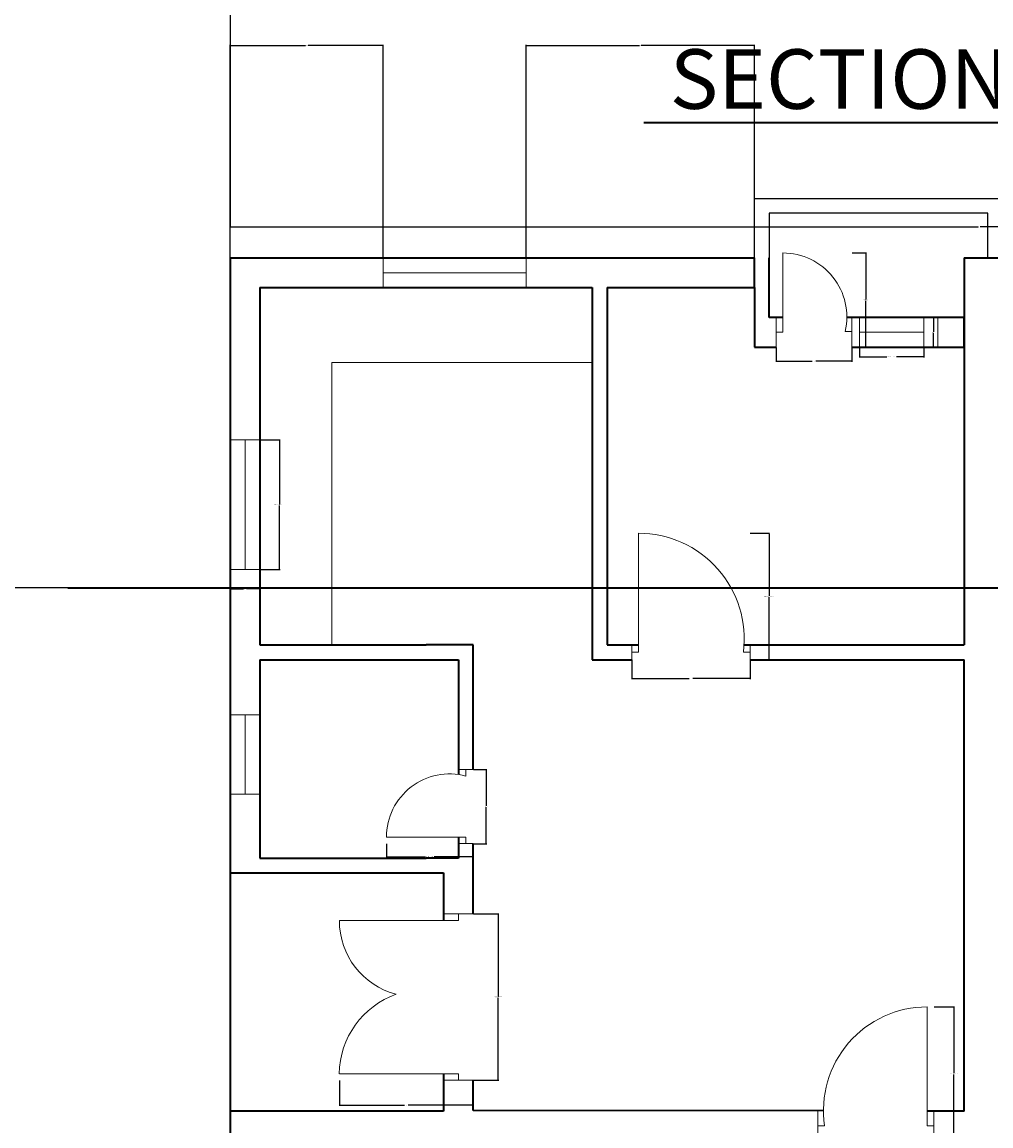
# Model space of a CAD drawing. Units: inches. Extents: x 2250 to 3629, y 982 to 2740.
# Tile 8 of 12: x 2918 to 3211, y 1785 to 2119. Entities that reach past the tile are written whole.
import ezdxf

# ---------------------------------------------------------------- set-up
doc = ezdxf.new("R2010")
doc.units = ezdxf.units.IN
for name, color, linetype, lineweight in [('A-ANNO-DIMS', 2, 'Continuous', 18), ('A-ANNO-SYMB', 7, 'Continuous', 35), ('A-ANNO-TITL', 7, 'Continuous', 35), ('A-DOOR', 3, 'Continuous', 18), ('A-FLOR-DECK', 7, 'Continuous', 25), ('A-FLOR-FIXT', 9, 'Continuous', 18), ('A-GLAZ', 4, 'Continuous', 18), ('A-WALL', 7, 'Continuous', 35)]:
    doc.layers.add(name, color=color, linetype=linetype, lineweight=lineweight)
doc.styles.get("Standard").update_dxf_attribs({"font": 'arial.ttf'})
doc.dimstyles.get("Standard").update_dxf_attribs({"dimtxt": 0.18, "dimasz": 0.18, "dimexe": 0.18, "dimexo": 0.0625, "dimgap": 0.09, "dimtad": 0, "dimtih": 1, "dimtoh": 1, "dimdec": 4, "dimzin": 0, "dimdsep": 46, "dimtxsty": 'Standard', "dimcen": 0.09, "dimadec": 0, "dimazin": 0, "dimtfac": 1, "dimtdec": 4, "dimtofl": 0, "dimtmove": 0, "dimatfit": 3, "dimfxl": 1, "dimtolj": 1, "dimtzin": 0, "dimarcsym": 0})

# ---------------------------------------------------------------- blocks, each defined once
blk = doc.blocks.new('DR-36-BED-NW')
for p, q in [((2, 2.25), (2, 38.25)), ((0, 4.5), (0, 0)), ((35.76, 4.5), (35.76, 0)), ((0, 0), (0, 2.25)), ((0, 2.25), (2, 2.25)), ((35.76, 2.25), (33.76, 2.25)), ((35.76, 0), (35.76, 2.25))]:
    blk.add_line(p, q)
blk.add_arc((2, 6.24), 32.01, 352.8376, 90)
blk = doc.blocks.new('DR-24-DECK-NW')
for p, q in [((2, 4.5), (2, 28.5)), ((0, 9), (0, 0)), ((22.88, 0), (22.88, 9)), ((22.88, 9), (22.88, 4.79)), ((0, 0), (0, 4.5)), ((0, 4.5), (2, 4.5)), ((22.88, 4.79), (20.88, 4.79))]:
    blk.add_line(p, q)
blk.add_arc((2, 9.13), 19.37, 347.0543, 90)
blk = doc.blocks.new('DR-72-DECK-WEST-N')
for p, q in [((31.5, 50.33), (40.5, 50.33)), ((40.5, 50.33), (36, 50.33)), ((36, 50.33), (36, 48.33)), ((36, 48.33), (0, 48.33)), ((36, 2), (0, 2)), ((36, 0), (36, 2)), ((31.5, 0), (40.5, 0)), ((40.5, 0), (36, 0))]:
    blk.add_line(p, q)
for centre, radius, start, end in [((23.09, 48.33), 23.09, 180, 255.1842), ((25.75, 1.72), 25.76, 109.4277, 179.3734)]:
    blk.add_arc(centre, radius, start, end)
blk = doc.blocks.new('DR-24-BATH-NW')
for p, q in [((21.75, 22.45), (26.25, 22.45)), ((26.25, 22.45), (24, 22.45)), ((24, 22.45), (24, 20.45)), ((24, 2), (0, 2)), ((24, 0), (24, 2)), ((21.75, 0), (26.25, 0)), ((26.25, 0), (24, 0))]:
    blk.add_line(p, q)
blk.add_arc((19.09, 2), 19.09, 75.0892, 180)
blk = doc.blocks.new('DR-36-ENTRY-NW')
for p, q in [((33.05, 4.5), (33.05, 40.5)), ((0, 9.04), (0, 0)), ((35.05, 9.01), (35.05, 0)), ((0, 0), (0, 4.52)), ((0, 4.52), (2, 4.52)), ((35.05, 4.5), (33.05, 4.5)), ((35.05, 0), (35.05, 4.5))]:
    blk.add_line(p, q)
blk.add_arc((33.05, 9.12), 31.39, 90, 188.415)
blk = doc.blocks.new('WIN-DECK-NW')
for p, q in [((0.07, 4.5), (0.07, 9)), ((0.07, 9), (0.07, 1.12)), ((19.52, 9), (19.52, 0)), ((19.52, 4.5), (0.07, 4.5)), ((19.52, 0), (19.52, 4.5)), ((0.07, 1.12), (0, 0))]:
    blk.add_line(p, q)
blk = doc.blocks.new('WIN-KITCHEN-NW-A')
for p, q in [((0, 9), (0, 0)), ((43.24, 4.5), (43.24, 9)), ((43.24, 9), (43.24, 0)), ((0, 4.5), (43.24, 4.5))]:
    blk.add_line(p, q)
blk = doc.blocks.new('WIN-KITCHEN-NW-B')
for p, q in [((0, 39.2), (9, 39.2)), ((4.5, 0), (4.5, 39.2)), ((9, 0), (0, 0)), ((0, 0), (4.5, 0))]:
    blk.add_line(p, q)
blk = doc.blocks.new('WIN-24-BATH-NW')
for p, q in [((9, 24), (0, 24)), ((0, 24), (4.5, 24)), ((4.5, 24), (4.5, 0)), ((9, 0), (0, 0)), ((4.5, 0), (9, 0))]:
    blk.add_line(p, q)
blk = doc.blocks.new('*D85')
at = {"layer": 'A-ANNO-DIMS', "color": 0, "lineweight": -2, "transparency": 16777216}
for p, q in [((3171.49, 2020.67), (3171.49, 2017.63)), ((3191.01, 2020.67), (3191.01, 2017.63)), ((3171.67, 2017.81), (3179.76, 2017.81)), ((3190.83, 2017.81), (3182.75, 2017.81))]:
    blk.add_line(p, q, dxfattribs=at)
at = {"layer": 'A-ANNO-DIMS', "color": 0, "transparency": 16777216}
for points in [[(3171.67, 2017.84), (3171.67, 2017.78), (3171.49, 2017.81)], [(3190.83, 2017.84), (3190.83, 2017.78), (3191.01, 2017.81)]]:
    blk.add_solid(points, dxfattribs=at)
at = {"layer": 'Defpoints', "color": 0, "transparency": 16777216}
for p in [(3171.49, 2020.74), (3191.01, 2020.74), (3191.01, 2017.81)]:
    blk.add_point(p, dxfattribs=at)
at = {"layer": 'A-ANNO-DIMS', "color": 0, "transparency": 16777216, "insert": (3181.25, 2017.81), "char_height": 0.18, "attachment_point": 5}
blk.add_mtext('\\A1;DECK WINDOW 20 TYP.', dxfattribs=at)
blk = doc.blocks.new('*D86')
at = {"layer": 'A-ANNO-DIMS', "color": 0, "lineweight": -2, "transparency": 16777216}
for p, q in [((3191.07, 2029.74), (3194.12, 2029.74)), ((3193.94, 2029.56), (3193.94, 2025.42)), ((3193.94, 2020.92), (3193.94, 2025.05)), ((3191.07, 2020.74), (3194.12, 2020.74))]:
    blk.add_line(p, q, dxfattribs=at)
at = {"layer": 'A-ANNO-DIMS', "color": 0, "transparency": 16777216}
for points in [[(3193.91, 2029.56), (3193.97, 2029.56), (3193.94, 2029.74)], [(3193.91, 2020.92), (3193.97, 2020.92), (3193.94, 2020.74)]]:
    blk.add_solid(points, dxfattribs=at)
at = {"layer": 'Defpoints', "color": 0, "transparency": 16777216}
for p in [(3191.01, 2029.74), (3193.94, 2029.74), (3191.01, 2020.74)]:
    blk.add_point(p, dxfattribs=at)
at = {"layer": 'A-ANNO-DIMS', "color": 0, "transparency": 16777216, "insert": (3193.94, 2025.24), "char_height": 0.18, "attachment_point": 5}
blk.add_mtext('\\A1;9 TYP.', dxfattribs=at)
blk = doc.blocks.new('*D89')
at = {"layer": 'A-ANNO-DIMS', "color": 0, "lineweight": -2, "transparency": 16777216}
for p, q in [((2990.29, 1992.69), (2996.29, 1992.69)), ((2996.11, 1992.51), (2996.11, 1973.27)), ((2996.11, 1953.67), (2996.11, 1972.9)), ((2990.29, 1953.49), (2996.29, 1953.49))]:
    blk.add_line(p, q, dxfattribs=at)
at = {"layer": 'A-ANNO-DIMS', "color": 0, "transparency": 16777216}
for points in [[(2996.08, 1992.51), (2996.14, 1992.51), (2996.11, 1992.69)], [(2996.08, 1953.67), (2996.14, 1953.67), (2996.11, 1953.49)]]:
    blk.add_solid(points, dxfattribs=at)
at = {"layer": 'Defpoints', "color": 0, "transparency": 16777216}
for p in [(2990.23, 1992.69), (2996.11, 1992.69), (2990.23, 1953.49)]:
    blk.add_point(p, dxfattribs=at)
at = {"layer": 'A-ANNO-DIMS', "color": 0, "transparency": 16777216, "insert": (2996.11, 1973.09), "char_height": 0.18, "attachment_point": 5}
blk.add_mtext('\\A1;KITCHEN WINDOW 39 TYP.', dxfattribs=at)
blk = doc.blocks.new('*D90')
at = {"layer": 'A-ANNO-DIMS', "color": 0, "lineweight": -2, "transparency": 16777216}
for p, q in [((2981.23, 1953.42), (2981.23, 1947.43)), ((2990.23, 1953.42), (2990.23, 1947.43)), ((2981.41, 1947.61), (2985.27, 1947.61)), ((2990.05, 1947.61), (2986.18, 1947.61))]:
    blk.add_line(p, q, dxfattribs=at)
at = {"layer": 'A-ANNO-DIMS', "color": 0, "transparency": 16777216}
for points in [[(2981.41, 1947.64), (2981.41, 1947.58), (2981.23, 1947.61)], [(2990.05, 1947.64), (2990.05, 1947.58), (2990.23, 1947.61)]]:
    blk.add_solid(points, dxfattribs=at)
at = {"layer": 'Defpoints', "color": 0, "transparency": 16777216}
for p in [(2981.23, 1953.49), (2990.23, 1953.49), (2990.23, 1947.61)]:
    blk.add_point(p, dxfattribs=at)
at = {"layer": 'A-ANNO-DIMS', "color": 0, "transparency": 16777216, "insert": (2985.73, 1947.61), "char_height": 0.18, "attachment_point": 5}
blk.add_mtext('\\A1;9 TYP.', dxfattribs=at)
blk = doc.blocks.new('*D103')
at = {"layer": 'A-ANNO-DIMS', "color": 0, "lineweight": -2, "transparency": 16777216}
for p, q in [((3138.49, 1964.49), (3144.35, 1964.49)), ((3144.17, 1964.31), (3144.17, 1945.54)), ((3144.17, 1926.42), (3144.17, 1945.18)), ((3138.49, 1926.24), (3144.35, 1926.24))]:
    blk.add_line(p, q, dxfattribs=at)
at = {"layer": 'A-ANNO-DIMS', "color": 0, "transparency": 16777216}
for points in [[(3144.14, 1964.31), (3144.2, 1964.31), (3144.17, 1964.49)], [(3144.14, 1926.42), (3144.2, 1926.42), (3144.17, 1926.24)]]:
    blk.add_solid(points, dxfattribs=at)
at = {"layer": 'Defpoints', "color": 0, "transparency": 16777216}
for p in [(3138.43, 1964.49), (3144.17, 1964.49), (3138.43, 1926.24)]:
    blk.add_point(p, dxfattribs=at)
at = {"layer": 'A-ANNO-DIMS', "color": 0, "transparency": 16777216, "insert": (3144.17, 1945.36), "char_height": 0.18, "attachment_point": 5}
blk.add_mtext('\\A1;BEDROOM DOOR 38 TYP.', dxfattribs=at)
blk = doc.blocks.new('*D104')
at = {"layer": 'A-ANNO-DIMS', "color": 0, "lineweight": -2, "transparency": 16777216}
for p, q in [((3102.67, 1926.17), (3102.67, 1920.32)), ((3138.43, 1926.17), (3138.43, 1920.32)), ((3102.85, 1920.5), (3120.02, 1920.5)), ((3138.25, 1920.5), (3121.08, 1920.5))]:
    blk.add_line(p, q, dxfattribs=at)
at = {"layer": 'A-ANNO-DIMS', "color": 0, "transparency": 16777216}
for points in [[(3102.85, 1920.53), (3102.85, 1920.47), (3102.67, 1920.5)], [(3138.25, 1920.53), (3138.25, 1920.47), (3138.43, 1920.5)]]:
    blk.add_solid(points, dxfattribs=at)
at = {"layer": 'Defpoints', "color": 0, "transparency": 16777216}
for p in [(3102.67, 1926.24), (3138.43, 1926.24), (3138.43, 1920.5)]:
    blk.add_point(p, dxfattribs=at)
at = {"layer": 'A-ANNO-DIMS', "color": 0, "transparency": 16777216, "insert": (3120.55, 1920.5), "char_height": 0.18, "attachment_point": 5}
blk.add_mtext('\\A1;36 TYP.', dxfattribs=at)
blk = doc.blocks.new('*D105')
at = {"layer": 'A-ANNO-DIMS', "color": 0, "lineweight": -2, "transparency": 16777216}
for p, q in [((3169.27, 2049.24), (3173.67, 2049.24)), ((3173.49, 2049.06), (3173.49, 2035.17)), ((3173.49, 2020.92), (3173.49, 2034.8)), ((3169.27, 2020.74), (3173.67, 2020.74))]:
    blk.add_line(p, q, dxfattribs=at)
at = {"layer": 'A-ANNO-DIMS', "color": 0, "transparency": 16777216}
for points in [[(3173.46, 2049.06), (3173.52, 2049.06), (3173.49, 2049.24)], [(3173.46, 2020.92), (3173.52, 2020.92), (3173.49, 2020.74)]]:
    blk.add_solid(points, dxfattribs=at)
at = {"layer": 'Defpoints', "color": 0, "transparency": 16777216}
for p in [(3169.21, 2049.24), (3173.49, 2049.24), (3169.21, 2020.74)]:
    blk.add_point(p, dxfattribs=at)
at = {"layer": 'A-ANNO-DIMS', "color": 0, "transparency": 16777216, "insert": (3173.49, 2034.99), "char_height": 0.18, "attachment_point": 5}
blk.add_mtext('\\A1;DECK DOOR 29 TYP.', dxfattribs=at)
blk = doc.blocks.new('*D106')
at = {"layer": 'A-ANNO-DIMS', "color": 0, "lineweight": -2, "transparency": 16777216}
for p, q in [((3146.34, 2020.67), (3146.34, 2016.28)), ((3169.21, 2020.67), (3169.21, 2016.28)), ((3146.52, 2016.46), (3157.24, 2016.46)), ((3169.03, 2016.46), (3158.3, 2016.46))]:
    blk.add_line(p, q, dxfattribs=at)
at = {"layer": 'A-ANNO-DIMS', "color": 0, "transparency": 16777216}
for points in [[(3146.52, 2016.49), (3146.52, 2016.43), (3146.34, 2016.46)], [(3169.03, 2016.49), (3169.03, 2016.43), (3169.21, 2016.46)]]:
    blk.add_solid(points, dxfattribs=at)
at = {"layer": 'Defpoints', "color": 0, "transparency": 16777216}
for p in [(3146.34, 2020.74), (3169.21, 2020.74), (3169.21, 2016.46)]:
    blk.add_point(p, dxfattribs=at)
at = {"layer": 'A-ANNO-DIMS', "color": 0, "transparency": 16777216, "insert": (3157.77, 2016.46), "char_height": 0.18, "attachment_point": 5}
blk.add_mtext('\\A1;23 TYP.', dxfattribs=at)
blk = doc.blocks.new('*D107')
at = {"layer": 'A-ANNO-DIMS', "color": 0, "lineweight": -2, "transparency": 16777216}
for p, q in [((3054.79, 1849.36), (3062.46, 1849.36)), ((3062.28, 1849.18), (3062.28, 1824.38)), ((3062.28, 1799.21), (3062.28, 1824.01)), ((3054.79, 1799.03), (3062.46, 1799.03))]:
    blk.add_line(p, q, dxfattribs=at)
at = {"layer": 'A-ANNO-DIMS', "color": 0, "transparency": 16777216}
for points in [[(3062.25, 1849.18), (3062.31, 1849.18), (3062.28, 1849.36)], [(3062.25, 1799.21), (3062.31, 1799.21), (3062.28, 1799.03)]]:
    blk.add_solid(points, dxfattribs=at)
at = {"layer": 'Defpoints', "color": 0, "transparency": 16777216}
for p in [(3054.73, 1849.36), (3062.28, 1849.36), (3054.73, 1799.03)]:
    blk.add_point(p, dxfattribs=at)
at = {"layer": 'A-ANNO-DIMS', "color": 0, "transparency": 16777216, "insert": (3062.28, 1824.2), "char_height": 0.18, "attachment_point": 5}
blk.add_mtext('\\A1;DECK DOOR 50 TYP.', dxfattribs=at)
blk = doc.blocks.new('*D108')
at = {"layer": 'A-ANNO-DIMS', "color": 0, "lineweight": -2, "transparency": 16777216}
for p, q in [((3014.23, 1798.97), (3014.23, 1791.3)), ((3054.73, 1798.97), (3054.73, 1791.3)), ((3014.41, 1791.48), (3033.95, 1791.48)), ((3054.55, 1791.48), (3035.01, 1791.48))]:
    blk.add_line(p, q, dxfattribs=at)
at = {"layer": 'A-ANNO-DIMS', "color": 0, "transparency": 16777216}
for points in [[(3014.41, 1791.51), (3014.41, 1791.45), (3014.23, 1791.48)], [(3054.55, 1791.51), (3054.55, 1791.45), (3054.73, 1791.48)]]:
    blk.add_solid(points, dxfattribs=at)
at = {"layer": 'Defpoints', "color": 0, "transparency": 16777216}
for p in [(3014.23, 1799.03), (3054.73, 1799.03), (3054.73, 1791.48)]:
    blk.add_point(p, dxfattribs=at)
at = {"layer": 'A-ANNO-DIMS', "color": 0, "transparency": 16777216, "insert": (3034.48, 1791.48), "char_height": 0.18, "attachment_point": 5}
blk.add_mtext('\\A1;41 TYP.', dxfattribs=at)
blk = doc.blocks.new('*D109')
at = {"layer": 'A-ANNO-DIMS', "color": 0, "lineweight": -2, "transparency": 16777216}
for p, q in [((3028.48, 1870.53), (3028.48, 1866.48)), ((3054.73, 1870.53), (3054.73, 1866.48)), ((3028.66, 1866.66), (3040.3, 1866.66)), ((3054.55, 1866.66), (3042.91, 1866.66))]:
    blk.add_line(p, q, dxfattribs=at)
at = {"layer": 'A-ANNO-DIMS', "color": 0, "transparency": 16777216}
for points in [[(3028.66, 1866.69), (3028.66, 1866.63), (3028.48, 1866.66)], [(3054.55, 1866.69), (3054.55, 1866.63), (3054.73, 1866.66)]]:
    blk.add_solid(points, dxfattribs=at)
at = {"layer": 'Defpoints', "color": 0, "transparency": 16777216}
for p in [(3028.48, 1870.59), (3054.73, 1870.59), (3054.73, 1866.66)]:
    blk.add_point(p, dxfattribs=at)
at = {"layer": 'A-ANNO-DIMS', "color": 0, "transparency": 16777216, "insert": (3041.6, 1866.66), "char_height": 0.18, "attachment_point": 5}
blk.add_mtext('\\A1;BATH DOOR 26 TYP.', dxfattribs=at)
blk = doc.blocks.new('*D110')
at = {"layer": 'A-ANNO-DIMS', "color": 0, "lineweight": -2, "transparency": 16777216}
for p, q in [((3054.79, 1893.04), (3058.84, 1893.04)), ((3058.66, 1892.86), (3058.66, 1882)), ((3058.66, 1870.77), (3058.66, 1881.64)), ((3054.79, 1870.59), (3058.84, 1870.59))]:
    blk.add_line(p, q, dxfattribs=at)
at = {"layer": 'A-ANNO-DIMS', "color": 0, "transparency": 16777216}
for points in [[(3058.63, 1892.86), (3058.69, 1892.86), (3058.66, 1893.04)], [(3058.63, 1870.77), (3058.69, 1870.77), (3058.66, 1870.59)]]:
    blk.add_solid(points, dxfattribs=at)
at = {"layer": 'Defpoints', "color": 0, "transparency": 16777216}
for p in [(3054.73, 1893.04), (3058.66, 1893.04), (3054.73, 1870.59)]:
    blk.add_point(p, dxfattribs=at)
at = {"layer": 'A-ANNO-DIMS', "color": 0, "transparency": 16777216, "insert": (3058.66, 1881.82), "char_height": 0.18, "attachment_point": 5}
blk.add_mtext('\\A1;22 TYP.', dxfattribs=at)
blk = doc.blocks.new('*D137')
at = {"layer": 'A-ANNO-DIMS', "color": 0, "lineweight": -2, "transparency": 16777216}
for p, q in [((3194.07, 1821.24), (3200.27, 1821.24)), ((3200.09, 1821.06), (3200.09, 1801.17)), ((3200.09, 1780.92), (3200.09, 1800.8)), ((3194.07, 1780.74), (3200.27, 1780.74))]:
    blk.add_line(p, q, dxfattribs=at)
at = {"layer": 'A-ANNO-DIMS', "color": 0, "transparency": 16777216}
for points in [[(3200.06, 1821.06), (3200.12, 1821.06), (3200.09, 1821.24)], [(3200.06, 1780.92), (3200.12, 1780.92), (3200.09, 1780.74)]]:
    blk.add_solid(points, dxfattribs=at)
at = {"layer": 'Defpoints', "color": 0, "transparency": 16777216}
for p in [(3194.01, 1821.24), (3200.09, 1821.24), (3194.01, 1780.74)]:
    blk.add_point(p, dxfattribs=at)
at = {"layer": 'A-ANNO-DIMS', "color": 0, "transparency": 16777216, "insert": (3200.09, 1800.99), "char_height": 0.18, "attachment_point": 5}
blk.add_mtext('\\A1;ENTRY DOOR 41 TYP.', dxfattribs=at)
blk = doc.blocks.new('*D172')
at = {"layer": 'A-ANNO-DIMS', "color": 0, "lineweight": -2, "transparency": 16777216}
for p, q in [((3433.02, 2070.24), (3541.21, 2070.24)), ((3541.03, 2070.06), (3541.03, 1664.67)), ((3541.03, 1258.92), (3541.03, 1664.3)), ((3059.29, 1258.74), (3541.21, 1258.74))]:
    blk.add_line(p, q, dxfattribs=at)
at = {"layer": 'A-ANNO-DIMS', "color": 0, "transparency": 16777216}
for points in [[(3541, 2070.06), (3541.06, 2070.06), (3541.03, 2070.24)], [(3541, 1258.92), (3541.06, 1258.92), (3541.03, 1258.74)]]:
    blk.add_solid(points, dxfattribs=at)
at = {"layer": 'Defpoints', "color": 0, "transparency": 16777216}
for p in [(3432.96, 2070.24), (3541.03, 2070.24), (3059.23, 1258.74)]:
    blk.add_point(p, dxfattribs=at)
at = {"layer": 'A-ANNO-DIMS', "color": 0, "transparency": 16777216, "insert": (3541.03, 1664.49), "char_height": 0.18, "attachment_point": 5}
blk.add_mtext('\\A1;811.5', dxfattribs=at)
blk = doc.blocks.new('*D173')
at = {"layer": 'A-ANNO-DIMS', "color": 0, "lineweight": -2, "transparency": 16777216}
for p, q in [((2932.01, 1947.92), (2890.14, 1947.92)), ((2890.32, 1947.74), (2890.32, 1603.51)), ((2890.32, 1258.92), (2890.32, 1603.15)), ((2981.16, 1258.74), (2890.14, 1258.74))]:
    blk.add_line(p, q, dxfattribs=at)
at = {"layer": 'A-ANNO-DIMS', "color": 0, "transparency": 16777216}
for points in [[(2890.29, 1947.74), (2890.35, 1947.74), (2890.32, 1947.92)], [(2890.29, 1258.92), (2890.35, 1258.92), (2890.32, 1258.74)]]:
    blk.add_solid(points, dxfattribs=at)
at = {"layer": 'Defpoints', "color": 0, "transparency": 16777216}
for p in [(2932.07, 1947.92), (2890.32, 1258.74), (2981.23, 1258.74)]:
    blk.add_point(p, dxfattribs=at)
at = {"layer": 'A-ANNO-DIMS', "color": 0, "transparency": 16777216, "insert": (2890.32, 1603.33), "char_height": 0.18, "attachment_point": 5}
blk.add_mtext('\\A1;689.2', dxfattribs=at)
blk = doc.blocks.new('*D174')
at = {"layer": 'A-ANNO-DIMS', "color": 0, "lineweight": -2, "transparency": 16777216}
for p, q in [((2981.23, 2047.8), (2981.23, 2112.17)), ((2981.41, 2111.99), (3003.97, 2111.99)), ((3027.33, 2111.99), (3004.77, 2111.99)), ((3027.51, 2047.8), (3027.51, 2112.17))]:
    blk.add_line(p, q, dxfattribs=at)
at = {"layer": 'A-ANNO-DIMS', "color": 0, "transparency": 16777216}
for points in [[(2981.41, 2112.02), (2981.41, 2111.96), (2981.23, 2111.99)], [(3027.33, 2112.02), (3027.33, 2111.96), (3027.51, 2111.99)]]:
    blk.add_solid(points, dxfattribs=at)
at = {"layer": 'Defpoints', "color": 0, "transparency": 16777216}
for p in [(3027.51, 2111.99), (2981.23, 2047.74), (3027.51, 2047.74)]:
    blk.add_point(p, dxfattribs=at)
at = {"layer": 'A-ANNO-DIMS', "color": 0, "transparency": 16777216, "insert": (3004.37, 2111.99), "char_height": 0.18, "attachment_point": 5}
blk.add_mtext('\\A1;46.29', dxfattribs=at)
blk = doc.blocks.new('*D175')
at = {"layer": 'A-ANNO-DIMS', "color": 0, "lineweight": -2, "transparency": 16777216}
for p, q in [((3070.76, 2047.8), (3070.76, 2112.17)), ((3070.94, 2111.99), (3105.04, 2111.99)), ((3139.57, 2111.99), (3105.47, 2111.99)), ((3139.75, 2047.8), (3139.75, 2112.17))]:
    blk.add_line(p, q, dxfattribs=at)
at = {"layer": 'A-ANNO-DIMS', "color": 0, "transparency": 16777216}
for points in [[(3070.94, 2112.02), (3070.94, 2111.96), (3070.76, 2111.99)], [(3139.57, 2112.02), (3139.57, 2111.96), (3139.75, 2111.99)]]:
    blk.add_solid(points, dxfattribs=at)
at = {"layer": 'Defpoints', "color": 0, "transparency": 16777216}
for p in [(3139.75, 2111.99), (3070.76, 2047.74), (3139.75, 2047.74)]:
    blk.add_point(p, dxfattribs=at)
at = {"layer": 'A-ANNO-DIMS', "color": 0, "transparency": 16777216, "insert": (3105.25, 2111.99), "char_height": 0.18, "attachment_point": 5}
blk.add_mtext('\\A1;69', dxfattribs=at)
blk = doc.blocks.new('*D188')
at = {"layer": 'A-ANNO-DIMS', "color": 0, "lineweight": -2, "transparency": 16777216}
for p, q in [((2981.23, 2131.64), (2981.23, 2056.9)), ((3434.23, 2131.64), (3434.23, 2056.9)), ((2981.41, 2057.08), (3207.43, 2057.08)), ((3434.05, 2057.08), (3208.02, 2057.08))]:
    blk.add_line(p, q, dxfattribs=at)
at = {"layer": 'A-ANNO-DIMS', "color": 0, "transparency": 16777216}
for points in [[(2981.41, 2057.11), (2981.41, 2057.05), (2981.23, 2057.08)], [(3434.05, 2057.11), (3434.05, 2057.05), (3434.23, 2057.08)]]:
    blk.add_solid(points, dxfattribs=at)
at = {"layer": 'Defpoints', "color": 0, "transparency": 16777216}
for p in [(2981.23, 2131.7), (3434.23, 2131.7), (3434.23, 2057.08)]:
    blk.add_point(p, dxfattribs=at)
at = {"layer": 'A-ANNO-DIMS', "color": 0, "transparency": 16777216, "insert": (3207.73, 2057.08), "char_height": 0.18, "attachment_point": 5}
blk.add_mtext('\\A1;453', dxfattribs=at)

msp = doc.modelspace()

# ---------------------------------------------------------------- linework, layer by layer
at = {"layer": 'A-ANNO-SYMB'}
msp.add_line((2932.0741, 1947.9231), (3499.2778, 1947.9231), dxfattribs=at)
at = {"layer": 'A-ANNO-TITL'}
msp.add_line((3253.0344, 2088.5817), (3106.2899, 2088.5817), dxfattribs=at)
at = {"layer": 'A-FLOR-DECK'}
for p, q in [((3139.754, 2047.7354), (3139.754, 2065.7354)), ((3139.754, 2065.7354), (3214.8276, 2065.7354)), ((3210.3276, 2061.2354), (3144.254, 2061.2354)), ((3144.254, 2061.2354), (3144.254, 2046.3774)), ((3210.3276, 2047.7354), (3210.3276, 2061.2354)), ((3214.8276, 2047.7354), (3210.3276, 2047.7354))]:
    msp.add_line(p, q, dxfattribs=at)
at = {"layer": 'A-FLOR-FIXT'}
for p, q in [((3011.954, 1930.7354), (3011.954, 2016.1232)), ((3011.954, 2016.1232), (3090.7267, 2016.1232))]:
    msp.add_line(p, q, dxfattribs=at)
at = {"layer": 'A-GLAZ'}
msp.add_line((3195.2491, 2029.7354), (3195.2491, 2020.7354), dxfattribs=at)
at = {"layer": 'A-WALL'}
for p, q in [((2981.2267, 2047.7354), (2981.2267, 1276.7354)), ((2981.2267, 2047.7354), (3139.754, 2047.7354)), ((3139.754, 2038.7354), (3139.754, 2047.7354)), ((3144.254, 2029.7354), (3144.254, 2047.7354)), ((3203.2267, 2047.7354), (3203.2267, 1930.7354)), ((3203.2267, 2047.7354), (3356.2267, 2047.7354)), ((2990.2267, 2038.7354), (2990.2267, 1930.7354)), ((2990.2267, 2038.7354), (3090.7267, 2038.7354)), ((3090.7267, 2038.7354), (3090.7267, 1930.7354)), ((3095.2267, 2038.7354), (3095.2267, 1930.7354)), ((3095.2267, 2038.7354), (3139.754, 2038.7354)), ((3139.754, 2038.7354), (3139.754, 2020.7354)), ((3148.3361, 2029.7354), (3144.254, 2029.7354)), ((3203.2267, 2029.7354), (3167.7042, 2029.7354)), ((3203.2267, 2020.7354), (3203.2267, 2029.7354)), ((3139.754, 2020.7354), (3146.3361, 2020.7354)), ((3169.2123, 2020.7354), (3203.2267, 2020.7354)), ((2990.2267, 1930.7354), (3040.4767, 1930.7354)), ((3054.7267, 1930.7354), (3040.4767, 1930.7354)), ((3054.7267, 1893.0402), (3054.7267, 1930.7354)), ((3090.7267, 1930.7354), (3090.7267, 1926.2354)), ((3095.2267, 1930.7354), (3104.6684, 1930.7354)), ((3136.63, 1930.7354), (3203.2267, 1930.7354)), ((2990.2267, 1926.2354), (2990.2267, 1866.2354)), ((2990.2267, 1926.2354), (3040.4767, 1926.2354)), ((2990.2267, 1926.2354), (3050.2267, 1926.2354)), ((3050.2267, 1926.2354), (3050.2267, 1891.4965)), ((3090.7267, 1926.2354), (3102.6684, 1926.2354)), ((3138.4276, 1926.2354), (3203.2267, 1926.2354)), ((3138.4276, 1926.2354), (3203.2267, 1926.2354)), ((3203.2267, 1789.7354), (3203.2267, 1926.2354)), ((3050.2267, 1872.5947), (3050.2267, 1866.2354)), ((3054.7267, 1861.7354), (3054.7267, 1870.5947)), ((2990.2267, 1866.2354), (3040.4767, 1866.2354)), ((3050.2267, 1866.2354), (3040.4767, 1866.2354)), ((2981.2267, 1861.7354), (3040.4767, 1861.7354)), ((3040.4767, 1861.7354), (3045.7267, 1861.7354)), ((3045.7267, 1861.7354), (3045.7267, 1847.3616)), ((3054.7267, 1849.3616), (3054.7267, 1861.7354)), ((3045.7267, 1801.0299), (3045.7267, 1789.7354)), ((3054.7267, 1789.8827), (3054.7267, 1799.0299)), ((3045.7267, 1789.7354), (2981.2267, 1789.7354)), ((3160.6233, 1789.7777), (3054.7267, 1789.8827)), ((3203.2267, 1789.7354), (3192.0123, 1789.7465))]:
    msp.add_line(p, q, dxfattribs=at)

# ---------------------------------------------------------------- block references
at = {"layer": 'A-DOOR'}
for name, p in [('DR-24-DECK-NW', (3146.3365, 2020.735)), ('DR-36-BED-NW', (3102.6685, 1926.235)), ('DR-24-BATH-NW', (3028.4765, 1870.595)), ('DR-72-DECK-WEST-N', (3014.2265, 1799.03)), ('DR-36-ENTRY-NW', (3158.9615, 1780.735))]:
    msp.add_blockref(name, p, dxfattribs=at)
at = {"layer": 'A-GLAZ'}
for name, p in [('WIN-KITCHEN-NW-A', (3027.5145, 2038.735)), ('WIN-DECK-NW', (3171.4905, 2020.735)), ('WIN-KITCHEN-NW-B', (2981.2265, 1953.486)), ('WIN-24-BATH-NW', (2981.2265, 1885.572))]:
    msp.add_blockref(name, p, dxfattribs=at)

# ---------------------------------------------------------------- texts
at = {"layer": 'A-ANNO-TITL', "insert": (3114.1642, 2110.8168), "char_height": 18, "attachment_point": 1}
msp.add_mtext_dynamic_manual_height_columns('SECTION-A', width=241.677358, gutter_width=12.5, heights=[0], dxfattribs=at)

# ---------------------------------------------------------------- dimensions: what is measured, and where the dimension line sits
at = {"layer": 'A-ANNO-DIMS'}
for base, p1, p2, override, picture, middle in [((3434.2267, 2057.0817), (2981.2267, 2131.6999), (3434.2267, 2131.6999), {"dimdec": 0, "dimlfac": 1, "dimrnd": 0, "dimzin": 0, "dimdsep": 46, "dimlunit": 2}, '*D188', (3207.7267, 2057.0817)), ((3027.5144, 2111.9854), (2981.2267, 2047.7354), (3027.5144, 2047.7354), {"dimdec": 2, "dimlfac": 1, "dimrnd": 0, "dimzin": 0, "dimdsep": 46, "dimlunit": 2}, '*D174', (3004.3706, 2111.9854)), ((3139.754, 2111.9854), (3070.7557, 2047.7354), (3139.754, 2047.7354), {"dimdec": 0, "dimlfac": 1, "dimrnd": 0, "dimzin": 0, "dimdsep": 46, "dimlunit": 2}, '*D175', (3105.2548, 2111.9854))]:
    dim = msp.add_linear_dim(base=base, p1=p1, p2=p2, dimstyle='Standard', override=override, dxfattribs=at)
    dim.commit()
    dim.dimension.update_dxf_attribs({"geometry": picture, "text_midpoint": middle})
for base, p1, p2, picture, middle in [((3541.0278, 2070.2354), (3059.2267, 1258.7354), (3432.9579, 2070.2354), '*D172', (3541.0278, 1664.4854)), ((2890.3241, 1258.7354), (2932.0741, 1947.9231), (2981.2267, 1258.7354), '*D173', (2890.3241, 1603.3293))]:
    dim = msp.add_linear_dim(base=base, p1=p1, p2=p2, angle=90, dimstyle='Standard', override={"dimdec": 1, "dimlfac": 1, "dimrnd": 0, "dimzin": 0, "dimdsep": 46, "dimlunit": 2}, dxfattribs=at)
    dim.commit()
    dim.dimension.update_dxf_attribs({"geometry": picture, "text_midpoint": middle})
for base, p1, p2, text, picture, middle in [((3173.4873275614, 2049.2354249075), (3169.2123275614, 2020.7354249075), (3169.2123275614, 2049.2354249075), 'DECK DOOR <> TYP.', '*D105', (3173.4873275614, 2034.9854249075)), ((3193.9392, 2029.7354), (3191.0111, 2020.7354), (3191.0111, 2029.7354), '<> TYP.', '*D86', (3193.9392, 2025.2354)), ((2996.1067, 1992.6856), (2990.2267, 1953.4859), (2990.2267, 1992.6856), 'KITCHEN WINDOW <> TYP.', '*D89', (2996.1067, 1973.0857)), ((3144.1651, 1964.4854), (3138.4276, 1926.2354), (3138.4276, 1964.4854), 'BEDROOM DOOR <> TYP.', '*D103', (3144.1651, 1945.3604)), ((3058.6642, 1893.0402), (3054.7267, 1870.5947), (3054.7267, 1893.0402), '<> TYP.', '*D110', (3058.6642, 1881.8174)), ((3062.2765, 1849.3616), (3054.7267, 1799.0299), (3054.7267, 1849.3616), 'DECK DOOR <> TYP.', '*D107', (3062.2765, 1824.1958)), ((3200.088, 1821.24), (3194.0123, 1780.7354), (3194.0123, 1821.24), 'ENTRY DOOR <> TYP.', '*D137', (3200.088, 1800.9877))]:
    dim = msp.add_linear_dim(base=base, p1=p1, p2=p2, angle=90, text=text, dimstyle='Standard', override={"dimdec": 0, "dimlfac": 1, "dimrnd": 0, "dimzin": 0, "dimdsep": 46, "dimlunit": 2}, dxfattribs=at)
    dim.commit()
    dim.dimension.update_dxf_attribs({"geometry": picture, "text_midpoint": middle})
for base, p1, p2, text, picture, middle in [((3169.2123, 2016.4604), (3146.3361, 2020.7354), (3169.2123, 2020.7354), '<> TYP.', '*D106', (3157.7742, 2016.4604)), ((3191.0111, 2017.8073), (3171.4904, 2020.7354), (3191.0111, 2020.7354), 'DECK WINDOW <> TYP.', '*D85', (3181.2507, 2017.8073)), ((2990.2267, 1947.606), (2981.2267, 1953.4859), (2990.2267, 1953.4859), '<> TYP.', '*D90', (2985.7267, 1947.606)), ((3138.4276, 1920.4979), (3102.6684, 1926.2354), (3138.4276, 1926.2354), '<> TYP.', '*D104', (3120.548, 1920.4979)), ((3054.7267, 1866.6572), (3028.4767, 1870.5947), (3054.7267, 1870.5947), 'BATH DOOR <> TYP.', '*D109', (3041.6017, 1866.6572)), ((3054.726726419, 1791.4801890279), (3014.226726419, 1799.0299446323), (3054.726726419, 1799.0299446323), '<> TYP.', '*D108', (3034.476726419, 1791.4801890279))]:
    dim = msp.add_linear_dim(base=base, p1=p1, p2=p2, text=text, dimstyle='Standard', override={"dimdec": 0, "dimlfac": 1, "dimrnd": 0, "dimzin": 0, "dimdsep": 46, "dimlunit": 2}, dxfattribs=at)
    dim.commit()
    dim.dimension.update_dxf_attribs({"geometry": picture, "text_midpoint": middle})

doc.saveas('drawing.dxf')
